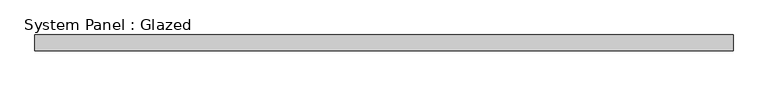
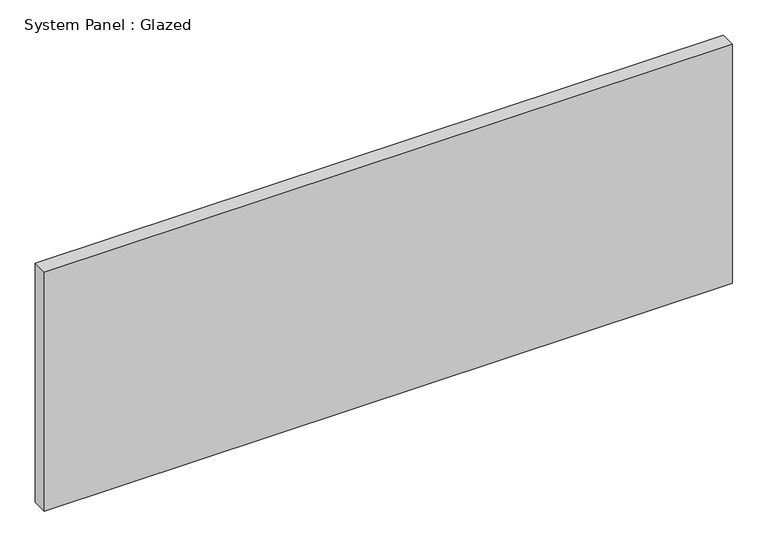
"""IFC4 building model written with IfcOpenShell, lengths in millimetres: plate geometry, System Panel : Glazed."""

from ifc_helpers import new_model, si_unit, origin, origin_with_axes, place, context, project, spatial, polyline, outline, extrude, source, transform, mapped, element, save


def system_panel_glazed_09ecb9ef(model_context):
    return source(origin(), model_context, "Body", "SweptSolid", [
        extrude(outline(polyline([(561.975, -44.45), (-561.975, -44.45), (-561.975, -19.05), (561.975, -19.05), (561.975, -44.45)])), origin_with_axes(), (0.0, 0.0, 1.0), 412.75),
    ])


if __name__ == "__main__":
    model = new_model("IFC4")
    model_context = context("Model", 3, world=origin())
    ifc_project = project(units=[si_unit("LENGTHUNIT", "METRE", prefix="MILLI")], contexts=[model_context])
    site = spatial("IfcSite", under=ifc_project)
    building = spatial("IfcBuilding", under=site)
    placement = place(None, origin())
    system_panel_glazed_shape = system_panel_glazed_09ecb9ef(model_context)
    element("IfcPlate", 1, ObjectType="System Panel : Glazed", at=placement, inside=building, context=model_context, shape_type="MappedRepresentation", body=[
        mapped(system_panel_glazed_shape, transform((0.0, 0.0, 0.0), x_axis=(1.0, 0.0, 0.0), y_axis=(0.0, 1.0, 0.0), z_axis=(0.0, 0.0, 1.0))),
    ])
    save(model, "model.ifc")

# Revit data of these elements
# Type "System Panel : Glazed"
#   Construction Type Id = "GSP4R"
#   Analytic Construction = "1/8 in Pilkington single glazing"
#   Visual Light Transmittance = 0.9
#   Solar Heat Gain Coefficient = 0.86
#   Heat Transfer Coefficient (U) = 1.18115 BTU/(h·ft²·°F)
#   Define Thermal Properties by = 1
# Element 1 (IfcPlate, "System Panel : Glazed")
#   Materials on its faces: "GARAGE PANEL"
# Materials
#   "GARAGE PANEL": class "Generic", colour RGB 120 120 120, transparency 0, Cost = 0
